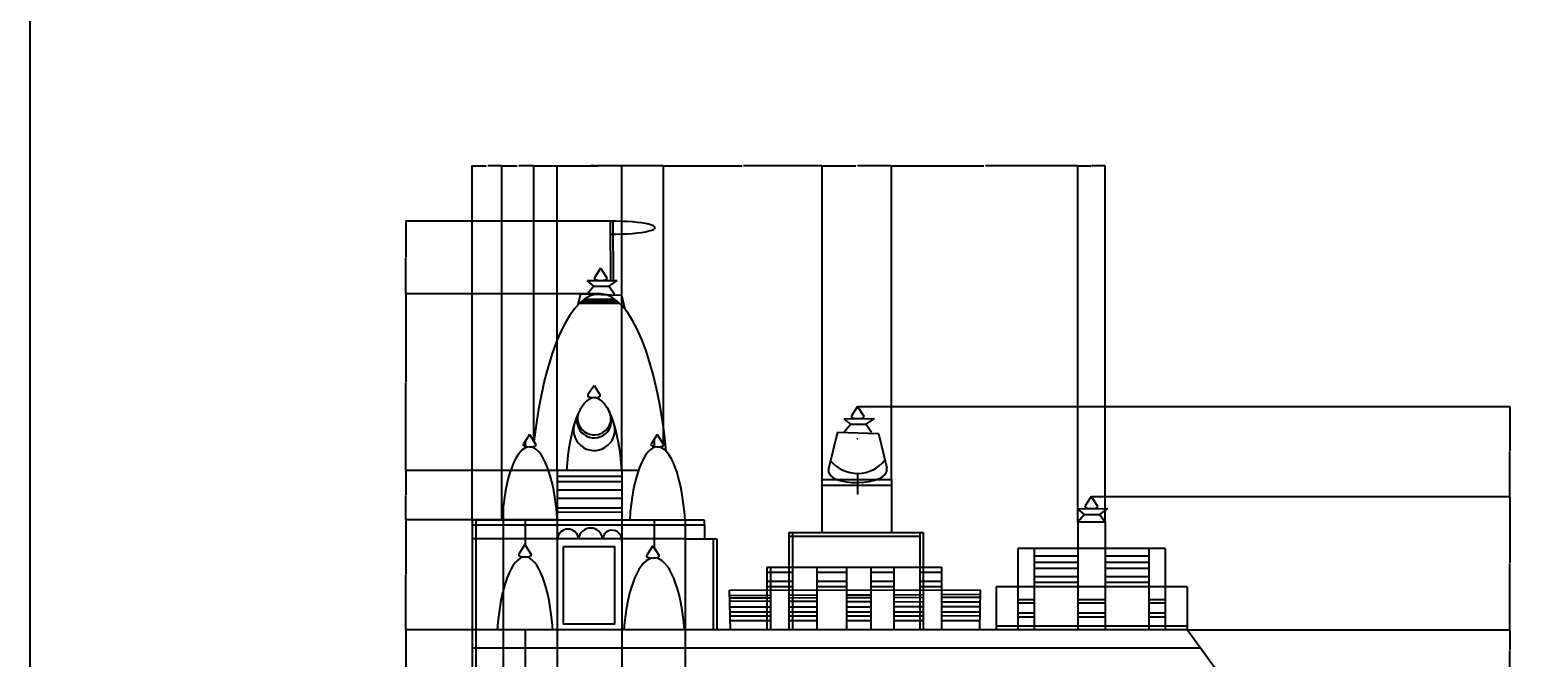
# Model space of a CAD drawing. Units: inches. Extents: x 386 to 107067, y -7 to 96314.
# Tile 2 of 10: x 386 to 1215, y 510 to 855. Entities that reach past the tile are written whole.
import ezdxf

# ---------------------------------------------------------------- set-up
doc = ezdxf.new("R2010")
doc.units = ezdxf.units.IN
doc.layers.add('A-ANNO-DIMS', color=2, linetype='Continuous', lineweight=18)
doc.layers.add('A-ELEV', color=7, linetype='Continuous', lineweight=25)
doc.styles.get("Standard").update_dxf_attribs({"font": 'arial.ttf'})
doc.dimstyles.get("Standard").update_dxf_attribs({"dimtxt": 0.18, "dimasz": 0.18, "dimexe": 0.18, "dimexo": 0.0625, "dimgap": 0.09, "dimtad": 0, "dimtih": 1, "dimtoh": 1, "dimdec": 4, "dimzin": 0, "dimdsep": 46, "dimtxsty": 'Standard', "dimcen": 0.09, "dimadec": 0, "dimazin": 0, "dimtfac": 1, "dimtdec": 4, "dimtofl": 0, "dimtmove": 0, "dimatfit": 3, "dimfxl": 1, "dimtolj": 1, "dimtzin": 0, "dimarcsym": 0})

# ---------------------------------------------------------------- blocks, each defined once
blk = doc.blocks.new('*D56')
at = {"layer": 'A-ANNO-DIMS', "color": 0, "lineweight": -2, "transparency": 16777216}
for p, q in [((628.96, 525.24), (592.35, 525.24)), ((592.53, 525.06), (592.53, 502.06)), ((592.53, 478.69), (592.53, 501.69)), ((728.96, 478.51), (592.35, 478.51))]:
    blk.add_line(p, q, dxfattribs=at)
at = {"layer": 'A-ANNO-DIMS', "color": 0, "transparency": 16777216}
for points in [[(592.5, 525.06), (592.56, 525.06), (592.53, 525.24)], [(592.5, 478.69), (592.56, 478.69), (592.53, 478.51)]]:
    blk.add_solid(points, dxfattribs=at)
at = {"layer": 'Defpoints', "color": 0, "transparency": 16777216}
for p in [(592.53, 525.24), (629.03, 525.24), (729.03, 478.51)]:
    blk.add_point(p, dxfattribs=at)
at = {"layer": 'A-ANNO-DIMS', "color": 0, "transparency": 16777216, "insert": (592.53, 501.88), "char_height": 0.18, "attachment_point": 5}
blk.add_mtext('\\A1;46.73', dxfattribs=at)
blk = doc.blocks.new('*D57')
at = {"layer": 'A-ANNO-DIMS', "color": 0, "lineweight": -2, "transparency": 16777216}
for p, q in [((628.96, 585.71), (592.35, 585.71)), ((592.53, 585.53), (592.53, 555.66)), ((592.53, 525.42), (592.53, 555.3)), ((628.96, 525.24), (592.35, 525.24))]:
    blk.add_line(p, q, dxfattribs=at)
at = {"layer": 'A-ANNO-DIMS', "color": 0, "transparency": 16777216}
for points in [[(592.5, 585.53), (592.56, 585.53), (592.53, 585.71)], [(592.5, 525.42), (592.56, 525.42), (592.53, 525.24)]]:
    blk.add_solid(points, dxfattribs=at)
at = {"layer": 'Defpoints', "color": 0, "transparency": 16777216}
for p in [(592.53, 585.71), (629.03, 585.71), (629.03, 525.24)]:
    blk.add_point(p, dxfattribs=at)
at = {"layer": 'A-ANNO-DIMS', "color": 0, "transparency": 16777216, "insert": (592.53, 555.48), "char_height": 0.18, "attachment_point": 5}
blk.add_mtext('\\A1;60.47', dxfattribs=at)
blk = doc.blocks.new('*D58')
at = {"layer": 'A-ANNO-DIMS', "color": 0, "lineweight": -2, "transparency": 16777216}
for p, q in [((675.71, 612.76), (592.35, 612.76)), ((592.53, 612.58), (592.53, 599.42)), ((592.53, 585.89), (592.53, 599.05)), ((675.71, 585.71), (592.35, 585.71))]:
    blk.add_line(p, q, dxfattribs=at)
at = {"layer": 'A-ANNO-DIMS', "color": 0, "transparency": 16777216}
for points in [[(592.5, 612.58), (592.56, 612.58), (592.53, 612.76)], [(592.5, 585.89), (592.56, 585.89), (592.53, 585.71)]]:
    blk.add_solid(points, dxfattribs=at)
at = {"layer": 'Defpoints', "color": 0, "transparency": 16777216}
for p in [(592.53, 612.76), (675.77, 612.76), (675.77, 585.71)]:
    blk.add_point(p, dxfattribs=at)
at = {"layer": 'A-ANNO-DIMS', "color": 0, "transparency": 16777216, "insert": (592.53, 599.24), "char_height": 0.18, "attachment_point": 5}
blk.add_mtext('\\A1;27.04', dxfattribs=at)
blk = doc.blocks.new('*D59')
at = {"layer": 'A-ANNO-DIMS', "color": 0, "lineweight": -2, "transparency": 16777216}
for p, q in [((699.85, 709.88), (592.35, 709.88)), ((592.53, 709.7), (592.53, 661.5)), ((592.53, 612.94), (592.53, 661.14)), ((675.71, 612.76), (592.35, 612.76))]:
    blk.add_line(p, q, dxfattribs=at)
at = {"layer": 'A-ANNO-DIMS', "color": 0, "transparency": 16777216}
for points in [[(592.5, 709.7), (592.56, 709.7), (592.53, 709.88)], [(592.5, 612.94), (592.56, 612.94), (592.53, 612.76)]]:
    blk.add_solid(points, dxfattribs=at)
at = {"layer": 'Defpoints', "color": 0, "transparency": 16777216}
for p in [(592.53, 709.88), (699.91, 709.88), (675.77, 612.76)]:
    blk.add_point(p, dxfattribs=at)
at = {"layer": 'A-ANNO-DIMS', "color": 0, "transparency": 16777216, "insert": (592.53, 661.32), "char_height": 0.18, "attachment_point": 5}
blk.add_mtext('\\A1;97.12', dxfattribs=at)
blk = doc.blocks.new('*D60')
at = {"layer": 'A-ANNO-DIMS', "color": 0, "lineweight": -2, "transparency": 16777216}
for p, q in [((704.79, 749.79), (592.35, 749.79)), ((592.53, 749.61), (592.53, 730.02)), ((592.53, 710.06), (592.53, 729.65)), ((699.85, 709.88), (592.35, 709.88))]:
    blk.add_line(p, q, dxfattribs=at)
at = {"layer": 'A-ANNO-DIMS', "color": 0, "transparency": 16777216}
for points in [[(592.5, 749.61), (592.56, 749.61), (592.53, 749.79)], [(592.5, 710.06), (592.56, 710.06), (592.53, 709.88)]]:
    blk.add_solid(points, dxfattribs=at)
at = {"layer": 'Defpoints', "color": 0, "transparency": 16777216}
for p in [(592.53, 749.79), (704.85, 749.79), (699.91, 709.88)]:
    blk.add_point(p, dxfattribs=at)
at = {"layer": 'A-ANNO-DIMS', "color": 0, "transparency": 16777216, "insert": (592.53, 729.84), "char_height": 0.18, "attachment_point": 5}
blk.add_mtext('\\A1;39.91', dxfattribs=at)
blk = doc.blocks.new('*D65')
at = {"layer": 'A-ANNO-DIMS', "color": 0, "lineweight": -2, "transparency": 16777216}
for p, q in [((1022.09, 525.24), (1199.71, 525.24)), ((1199.53, 525.06), (1199.53, 514.06)), ((1199.53, 502.69), (1199.53, 513.69)), ((1037.1, 502.51), (1199.71, 502.51))]:
    blk.add_line(p, q, dxfattribs=at)
at = {"layer": 'A-ANNO-DIMS', "color": 0, "transparency": 16777216}
for points in [[(1199.5, 525.06), (1199.56, 525.06), (1199.53, 525.24)], [(1199.5, 502.69), (1199.56, 502.69), (1199.53, 502.51)]]:
    blk.add_solid(points, dxfattribs=at)
at = {"layer": 'Defpoints', "color": 0, "transparency": 16777216}
for p in [(1022.03, 525.24), (1199.53, 525.24), (1037.04, 502.51)]:
    blk.add_point(p, dxfattribs=at)
at = {"layer": 'A-ANNO-DIMS', "color": 0, "transparency": 16777216, "insert": (1199.53, 513.88), "char_height": 0.18, "attachment_point": 5}
blk.add_mtext('\\A1;22.735', dxfattribs=at)
blk = doc.blocks.new('*D66')
at = {"layer": 'A-ANNO-DIMS', "color": 0, "lineweight": -2, "transparency": 16777216}
for p, q in [((969.43, 598.58), (1199.71, 598.58)), ((1199.53, 598.4), (1199.53, 562.09)), ((1199.53, 525.42), (1199.53, 561.73)), ((1022.09, 525.24), (1199.71, 525.24))]:
    blk.add_line(p, q, dxfattribs=at)
at = {"layer": 'A-ANNO-DIMS', "color": 0, "transparency": 16777216}
for points in [[(1199.5, 598.4), (1199.56, 598.4), (1199.53, 598.58)], [(1199.5, 525.42), (1199.56, 525.42), (1199.53, 525.24)]]:
    blk.add_solid(points, dxfattribs=at)
at = {"layer": 'Defpoints', "color": 0, "transparency": 16777216}
for p in [(969.37, 598.58), (1199.53, 598.58), (1022.03, 525.24)]:
    blk.add_point(p, dxfattribs=at)
at = {"layer": 'A-ANNO-DIMS', "color": 0, "transparency": 16777216, "insert": (1199.53, 561.91), "char_height": 0.18, "attachment_point": 5}
blk.add_mtext('\\A1;73.33', dxfattribs=at)
blk = doc.blocks.new('*D67')
at = {"layer": 'A-ANNO-DIMS', "color": 0, "lineweight": -2, "transparency": 16777216}
for p, q in [((840.97, 648.04), (1199.71, 648.04)), ((1199.53, 647.86), (1199.53, 623.49)), ((1199.53, 598.76), (1199.53, 623.13)), ((969.43, 598.58), (1199.71, 598.58))]:
    blk.add_line(p, q, dxfattribs=at)
at = {"layer": 'A-ANNO-DIMS', "color": 0, "transparency": 16777216}
for points in [[(1199.5, 647.86), (1199.56, 647.86), (1199.53, 648.04)], [(1199.5, 598.76), (1199.56, 598.76), (1199.53, 598.58)]]:
    blk.add_solid(points, dxfattribs=at)
at = {"layer": 'Defpoints', "color": 0, "transparency": 16777216}
for p in [(840.91, 648.04), (1199.53, 648.04), (969.37, 598.58)]:
    blk.add_point(p, dxfattribs=at)
at = {"layer": 'A-ANNO-DIMS', "color": 0, "transparency": 16777216, "insert": (1199.53, 623.31), "char_height": 0.18, "attachment_point": 5}
blk.add_mtext('\\A1;49.46', dxfattribs=at)
blk = doc.blocks.new('*D77')
at = {"layer": 'A-ANNO-DIMS', "color": 0, "lineweight": -2, "transparency": 16777216}
for p, q in [((629.03, 585.78), (629.03, 780.47)), ((629.21, 780.29), (636.73, 780.29)), ((645.16, 780.29), (637.64, 780.29)), ((645.34, 585.78), (645.34, 780.47))]:
    blk.add_line(p, q, dxfattribs=at)
at = {"layer": 'A-ANNO-DIMS', "color": 0, "transparency": 16777216}
for points in [[(629.21, 780.32), (629.21, 780.26), (629.03, 780.29)], [(645.16, 780.32), (645.16, 780.26), (645.34, 780.29)]]:
    blk.add_solid(points, dxfattribs=at)
at = {"layer": 'Defpoints', "color": 0, "transparency": 16777216}
for p in [(645.34, 780.29), (629.03, 585.71), (645.34, 585.71)]:
    blk.add_point(p, dxfattribs=at)
at = {"layer": 'A-ANNO-DIMS', "color": 0, "transparency": 16777216, "insert": (637.18, 780.29), "char_height": 0.18, "attachment_point": 5}
blk.add_mtext('\\A1;16.315', dxfattribs=at)
blk = doc.blocks.new('*D78')
at = {"layer": 'A-ANNO-DIMS', "color": 0, "lineweight": -2, "transparency": 16777216}
for p, q in [((645.34, 585.78), (645.34, 780.47)), ((645.52, 780.29), (653.68, 780.29)), ((662.74, 780.29), (654.59, 780.29)), ((662.92, 628.76), (662.92, 780.47))]:
    blk.add_line(p, q, dxfattribs=at)
at = {"layer": 'A-ANNO-DIMS', "color": 0, "transparency": 16777216}
for points in [[(645.52, 780.32), (645.52, 780.26), (645.34, 780.29)], [(662.74, 780.32), (662.74, 780.26), (662.92, 780.29)]]:
    blk.add_solid(points, dxfattribs=at)
at = {"layer": 'Defpoints', "color": 0, "transparency": 16777216}
for p in [(662.92, 780.29), (662.92, 628.7), (645.34, 585.71)]:
    blk.add_point(p, dxfattribs=at)
at = {"layer": 'A-ANNO-DIMS', "color": 0, "transparency": 16777216, "insert": (654.13, 780.29), "char_height": 0.18, "attachment_point": 5}
blk.add_mtext('\\A1;17.582', dxfattribs=at)
blk = doc.blocks.new('*D79')
at = {"layer": 'A-ANNO-DIMS', "color": 0, "lineweight": -2, "transparency": 16777216}
for p, q in [((662.92, 628.76), (662.92, 780.47)), ((663.1, 780.29), (698.14, 780.29)), ((733.96, 780.29), (698.93, 780.29)), ((734.14, 627.23), (734.14, 780.47))]:
    blk.add_line(p, q, dxfattribs=at)
at = {"layer": 'A-ANNO-DIMS', "color": 0, "transparency": 16777216}
for points in [[(663.1, 780.32), (663.1, 780.26), (662.92, 780.29)], [(733.96, 780.32), (733.96, 780.26), (734.14, 780.29)]]:
    blk.add_solid(points, dxfattribs=at)
at = {"layer": 'Defpoints', "color": 0, "transparency": 16777216}
for p in [(734.14, 780.29), (662.92, 628.7), (734.14, 627.16)]:
    blk.add_point(p, dxfattribs=at)
at = {"layer": 'A-ANNO-DIMS', "color": 0, "transparency": 16777216, "insert": (698.53, 780.29), "char_height": 0.18, "attachment_point": 5}
blk.add_mtext('\\A1;71.22', dxfattribs=at)
blk = doc.blocks.new('*D80')
at = {"layer": 'A-ANNO-DIMS', "color": 0, "lineweight": -2, "transparency": 16777216}
for p, q in [((734.14, 627.23), (734.14, 780.47)), ((734.32, 780.29), (777.34, 780.29)), ((821.15, 780.29), (778.13, 780.29)), ((821.33, 607.9), (821.33, 780.47))]:
    blk.add_line(p, q, dxfattribs=at)
at = {"layer": 'A-ANNO-DIMS', "color": 0, "transparency": 16777216}
for points in [[(734.32, 780.32), (734.32, 780.26), (734.14, 780.29)], [(821.15, 780.32), (821.15, 780.26), (821.33, 780.29)]]:
    blk.add_solid(points, dxfattribs=at)
at = {"layer": 'Defpoints', "color": 0, "transparency": 16777216}
for p in [(821.33, 780.29), (734.14, 627.16), (821.33, 607.84)]:
    blk.add_point(p, dxfattribs=at)
at = {"layer": 'A-ANNO-DIMS', "color": 0, "transparency": 16777216, "insert": (777.74, 780.29), "char_height": 0.18, "attachment_point": 5}
blk.add_mtext('\\A1;87.19', dxfattribs=at)
blk = doc.blocks.new('*D81')
at = {"layer": 'A-ANNO-DIMS', "color": 0, "lineweight": -2, "transparency": 16777216}
for p, q in [((821.33, 607.9), (821.33, 780.47)), ((821.51, 780.29), (839.95, 780.29)), ((859.32, 780.29), (840.88, 780.29)), ((859.5, 607.9), (859.5, 780.47))]:
    blk.add_line(p, q, dxfattribs=at)
at = {"layer": 'A-ANNO-DIMS', "color": 0, "transparency": 16777216}
for points in [[(821.51, 780.32), (821.51, 780.26), (821.33, 780.29)], [(859.32, 780.32), (859.32, 780.26), (859.5, 780.29)]]:
    blk.add_solid(points, dxfattribs=at)
at = {"layer": 'Defpoints', "color": 0, "transparency": 16777216}
for p in [(859.5, 780.29), (821.33, 607.84), (859.5, 607.84)]:
    blk.add_point(p, dxfattribs=at)
at = {"layer": 'A-ANNO-DIMS', "color": 0, "transparency": 16777216, "insert": (840.42, 780.29), "char_height": 0.18, "attachment_point": 5}
blk.add_mtext('\\A1;38.165', dxfattribs=at)
blk = doc.blocks.new('*D82')
at = {"layer": 'A-ANNO-DIMS', "color": 0, "lineweight": -2, "transparency": 16777216}
for p, q in [((859.5, 607.9), (859.5, 780.47)), ((859.68, 780.29), (910.31, 780.29)), ((961.85, 780.29), (911.22, 780.29)), ((962.03, 584.41), (962.03, 780.47))]:
    blk.add_line(p, q, dxfattribs=at)
at = {"layer": 'A-ANNO-DIMS', "color": 0, "transparency": 16777216}
for points in [[(859.68, 780.32), (859.68, 780.26), (859.5, 780.29)], [(961.85, 780.32), (961.85, 780.26), (962.03, 780.29)]]:
    blk.add_solid(points, dxfattribs=at)
at = {"layer": 'Defpoints', "color": 0, "transparency": 16777216}
for p in [(962.03, 780.29), (859.5, 607.84), (962.03, 584.35)]:
    blk.add_point(p, dxfattribs=at)
at = {"layer": 'A-ANNO-DIMS', "color": 0, "transparency": 16777216, "insert": (910.76, 780.29), "char_height": 0.18, "attachment_point": 5}
blk.add_mtext('\\A1;102.53', dxfattribs=at)
blk = doc.blocks.new('*D83')
at = {"layer": 'A-ANNO-DIMS', "color": 0, "lineweight": -2, "transparency": 16777216}
for p, q in [((962.03, 584.41), (962.03, 780.47)), ((962.21, 780.29), (969.31, 780.29)), ((976.85, 780.29), (969.74, 780.29)), ((977.03, 584.41), (977.03, 780.47))]:
    blk.add_line(p, q, dxfattribs=at)
at = {"layer": 'A-ANNO-DIMS', "color": 0, "transparency": 16777216}
for points in [[(962.21, 780.32), (962.21, 780.26), (962.03, 780.29)], [(976.85, 780.32), (976.85, 780.26), (977.03, 780.29)]]:
    blk.add_solid(points, dxfattribs=at)
at = {"layer": 'Defpoints', "color": 0, "transparency": 16777216}
for p in [(977.03, 780.29), (962.03, 584.35), (977.03, 584.35)]:
    blk.add_point(p, dxfattribs=at)
at = {"layer": 'A-ANNO-DIMS', "color": 0, "transparency": 16777216, "insert": (969.53, 780.29), "char_height": 0.18, "attachment_point": 5}
blk.add_mtext('\\A1;15', dxfattribs=at)
blk = doc.blocks.new('*D84')
at = {"layer": 'A-ANNO-DIMS', "color": 0, "lineweight": -2, "transparency": 16777216}
for p, q in [((675.77, 612.82), (675.77, 780.47)), ((675.95, 780.29), (693.06, 780.29)), ((711.09, 780.29), (693.98, 780.29)), ((711.27, 612.82), (711.27, 780.47))]:
    blk.add_line(p, q, dxfattribs=at)
at = {"layer": 'A-ANNO-DIMS', "color": 0, "transparency": 16777216}
for points in [[(675.95, 780.32), (675.95, 780.26), (675.77, 780.29)], [(711.09, 780.32), (711.09, 780.26), (711.27, 780.29)]]:
    blk.add_solid(points, dxfattribs=at)
at = {"layer": 'Defpoints', "color": 0, "transparency": 16777216}
for p in [(711.27, 780.29), (675.77, 612.76), (711.27, 612.76)]:
    blk.add_point(p, dxfattribs=at)
at = {"layer": 'A-ANNO-DIMS', "color": 0, "transparency": 16777216, "insert": (693.52, 780.29), "char_height": 0.18, "attachment_point": 5}
blk.add_mtext('\\A1;35.496', dxfattribs=at)
blk = doc.blocks.new('*D92')
at = {"layer": 'A-ANNO-DIMS', "color": 0, "lineweight": -2, "transparency": 16777216}
for p, q in [((840.73, 630.26), (840.91, 630.26)), ((840.82, 630.17), (840.82, 630.35)), ((841.11, 599.8), (841, 611.04)), ((841.29, 599.8), (841.11, 599.8))]:
    blk.add_line(p, q, dxfattribs=at)
at = {"layer": 'A-ANNO-DIMS', "color": 0, "transparency": 16777216}
blk.add_solid([(841.03, 611.04), (840.97, 611.04), (841, 611.22)], dxfattribs=at)
at = {"layer": 'Defpoints', "color": 0, "transparency": 16777216}
for p in [(840.82, 630.26), (841, 611.22)]:
    blk.add_point(p, dxfattribs=at)
at = {"layer": 'A-ANNO-DIMS', "color": 0, "transparency": 16777216, "insert": (841.76, 599.8), "char_height": 0.18, "attachment_point": 5}
blk.add_mtext('\\A1;R19.04', dxfattribs=at)

msp = doc.modelspace()

# ---------------------------------------------------------------- linework, layer by layer
at = {"layer": 'A-ELEV'}
for p, q in [((704.8536, 749.7917), (704.9724, 717.2635)), ((704.8536, 749.7917), (706.394, 749.7917)), ((706.394, 749.7917), (706.5128, 717.2692)), ((699.5858, 723.9778), (696.1948, 718.7355)), ((699.5858, 723.9778), (702.9769, 718.6076)), ((692.2048, 717.2169), (708.7758, 717.2774)), ((695.8991, 714.1217), (692.2048, 717.2169)), ((695.8991, 714.1217), (692.2387, 709.7528)), ((695.8991, 714.1217), (704.2155, 714.1217)), ((704.2155, 714.1217), (708.7758, 717.2774)), ((704.2155, 714.1217), (707.2387, 709.7528)), ((688.5858, 709.8864), (687.1082, 703.8169)), ((688.1023, 704.8132), (710.0986, 704.656)), ((688.5858, 709.8864), (711.0341, 709.0657)), ((689.0115, 705.6421), (709.2459, 705.4488)), ((689.9002, 706.3779), (708.1231, 706.3891)), ((690.6702, 706.957), (707.4109, 706.9256)), ((711.0341, 709.0657), (712.8802, 701.5787)), ((695.9971, 659.5746), (692.6061, 654.3323)), ((695.9971, 659.5746), (699.3882, 654.2045)), ((840.906, 648.0385), (837.515, 642.7962)), ((840.906, 648.0385), (844.2971, 642.6683)), ((833.5251, 641.2776), (850.096, 641.3382)), ((837.2193, 638.1824), (833.5251, 641.2776)), ((845.5357, 638.1824), (850.096, 641.3382)), ((660.5011, 632.5327), (657.1101, 627.2904)), ((660.5011, 632.5327), (663.8922, 627.1625)), ((730.7531, 632.5327), (727.3621, 627.2904)), ((730.7531, 632.5327), (734.1442, 627.1625)), ((829.906, 633.9471), (824.9784, 613.7052)), ((829.906, 633.9471), (852.3543, 633.1264)), ((837.2193, 638.1824), (833.5589, 633.8135)), ((837.2193, 638.1824), (845.5357, 638.1824)), ((845.5357, 638.1824), (848.5589, 633.8135)), ((852.3543, 633.1264), (857.0082, 614.2523)), ((658.0252, 628.7051), (658.0252, 625.1267)), ((729.0252, 629.8614), (729.0252, 625.4652)), ((720.3574, 612.7565), (671.0082, 612.7565)), ((675.7732, 612.7565), (675.7732, 451.5096)), ((675.7732, 609.7656), (711.2692, 609.7656)), ((711.2692, 606.5849), (675.7732, 606.5849)), ((711.2692, 612.7565), (711.2692, 322.5096)), ((821.3331, 578.7205), (821.3331, 607.8412)), ((821.3331, 607.8412), (859.4982, 607.8412)), ((859.4982, 607.8412), (859.4982, 578.7205)), ((675.7732, 602.1925), (711.2692, 602.1925)), ((711.2692, 597.4972), (675.7732, 597.4972)), ((821.3331, 604.8412), (859.4982, 604.8412)), ((969.3723, 598.5774), (965.9813, 593.3351)), ((969.3723, 598.5774), (972.7634, 593.2072)), ((646.0252, 593.3749), (646.0252, 274.5096)), ((675.7732, 592.3476), (711.2692, 592.3476)), ((711.2692, 589.9241), (675.7732, 589.7442)), ((961.9913, 591.8165), (978.5623, 591.877)), ((965.6856, 588.7213), (961.9913, 591.8165)), ((965.6856, 588.7213), (962.0252, 584.3524)), ((965.6856, 588.7213), (974.002, 588.7213)), ((974.002, 588.7213), (978.5623, 591.877)), ((974.002, 588.7213), (977.0252, 584.3524)), ((629.0252, 585.7146), (629.0252, 502.5096)), ((629.0252, 585.7146), (629.0252, 502.5096)), ((629.0252, 585.7146), (746.0252, 585.7146)), ((629.0252, 583.0118), (746.0252, 583.0118)), ((631.0252, 585.7146), (631.0252, 502.5096)), ((658.0252, 585.7146), (658.0252, 571.9741)), ((675.7732, 585.7146), (711.2692, 585.7146)), ((729.0252, 585.7146), (729.0252, 570.3474)), ((746.0252, 585.7146), (746.0252, 525.2442)), ((746.0252, 585.7146), (756.4861, 585.7146)), ((746.0252, 583.0118), (756.6362, 583.0118)), ((756.4861, 585.7146), (756.4861, 583.0118)), ((756.6362, 583.0118), (756.6362, 575.3263)), ((962.0252, 584.3524), (962.0252, 525.2442)), ((977.0252, 584.3524), (962.0252, 584.3524)), ((977.0252, 584.3524), (977.0252, 525.2442)), ((746.0252, 575.3263), (629.0252, 575.3263)), ((657.9695, 572.0623), (654.5785, 566.82)), ((657.9695, 572.0623), (661.3606, 566.6921)), ((746.0252, 575.3263), (763.5261, 575.3263)), ((761.3925, 575.3263), (761.3925, 525.2442)), ((763.5261, 575.3263), (763.5261, 525.2442)), ((803.0252, 578.7205), (803.0252, 525.2442)), ((803.0252, 578.7205), (875.0252, 578.7205)), ((803.0252, 576.7205), (875.0252, 576.7205)), ((805.0252, 578.7205), (805.0252, 525.2442)), ((875.0252, 578.7205), (875.0252, 525.2442)), ((875.0252, 578.7205), (877.0252, 578.7205)), ((877.0252, 578.7205), (877.0252, 525.2442)), ((728.3139, 571.4737), (724.923, 566.2314)), ((728.3139, 571.4737), (731.7051, 566.1036)), ((729.0252, 564.7745), (729.0252, 564.7473)), ((929.0252, 569.9003), (929.0252, 525.2442)), ((1010.0252, 569.9003), (929.0252, 569.9003)), ((938.0252, 569.9003), (938.0252, 525.2442)), ((938.0252, 565.8324), (962.0252, 565.8324)), ((977.0252, 565.8324), (1001.0252, 565.8324)), ((1001.0252, 569.9003), (1001.0252, 525.2442)), ((1010.0252, 569.9003), (1010.0252, 525.2442)), ((791.0252, 559.7024), (791.0252, 525.2442)), ((791.0252, 559.7024), (887.0252, 559.7024)), ((805.0252, 556.8053), (791.0252, 556.8053)), ((793.0252, 559.7024), (793.0252, 525.2442)), ((818.4886, 559.7024), (818.4886, 525.2442)), ((834.7141, 556.8053), (818.4886, 556.8053)), ((834.7141, 559.7024), (834.7141, 525.2442)), ((848.2048, 559.7024), (848.2048, 525.2442)), ((860.7841, 556.8053), (848.2048, 556.8053)), ((860.7841, 559.7024), (860.7841, 525.2442)), ((887.0252, 556.8053), (875.0252, 556.8053)), ((887.0252, 559.7024), (887.0252, 525.2442)), ((938.0252, 562.515), (962.0252, 562.515)), ((962.0252, 559.0468), (938.0252, 559.0468)), ((977.0252, 562.515), (1001.0252, 562.515)), ((1001.0252, 559.0468), (977.0252, 559.0468)), ((770.3702, 547.0345), (908.4441, 547.185)), ((791.0252, 551.9823), (805.0252, 551.9823)), ((791.0252, 549.1438), (805.0252, 549.1438)), ((818.4886, 551.9823), (834.7141, 551.9823)), ((818.4886, 549.1438), (834.7141, 549.1438)), ((848.2048, 551.9823), (860.7841, 551.9823)), ((848.2048, 549.1438), (860.7841, 549.1438)), ((875.0252, 551.9823), (887.0252, 551.9823)), ((875.0252, 549.1438), (887.0252, 549.1438)), ((908.1409, 525.2442), (908.4441, 547.185)), ((917.0252, 548.8243), (917.0252, 525.2442)), ((1022.0252, 548.8243), (917.0252, 548.8243)), ((938.0252, 554.5231), (962.0252, 554.5231)), ((962.0252, 551.2057), (938.0252, 551.2057)), ((977.0252, 554.5231), (1001.0252, 554.5231)), ((1001.0252, 551.2057), (977.0252, 551.2057)), ((1022.0252, 548.8243), (1022.0252, 525.2442)), ((771.0601, 525.2442), (770.3702, 547.0345)), ((770.4597, 544.2092), (793.0252, 544.3016)), ((793.0252, 542.7173), (770.5092, 542.6456)), ((793.0252, 540.8725), (770.5624, 540.9655)), ((803.0252, 544.3425), (818.4886, 544.4058)), ((818.4886, 542.7984), (803.0252, 542.7492)), ((818.4886, 540.767), (803.0252, 540.8311)), ((834.7141, 544.4723), (848.2048, 544.5275)), ((848.2048, 542.8931), (834.7141, 542.8501)), ((848.2048, 540.644), (834.7141, 540.6998)), ((860.7841, 544.579), (877.0252, 544.6455)), ((877.0252, 542.9849), (860.7841, 542.9332)), ((877.0252, 540.5246), (860.7841, 540.5919)), ((887.0252, 544.6865), (908.4107, 544.774)), ((908.3874, 543.0848), (887.0252, 543.0168)), ((908.3503, 540.3949), (887.0252, 540.4832)), ((929.0252, 541.8566), (938.0252, 541.8566)), ((938.0252, 539.8963), (929.0252, 539.8963)), ((962.0252, 541.8566), (977.0252, 541.8566)), ((977.0252, 539.8963), (962.0252, 539.8963)), ((1001.0252, 541.8566), (1010.0252, 541.8566)), ((1010.0252, 539.8963), (1001.0252, 539.8963)), ((770.6585, 537.9278), (793.0252, 537.9441)), ((770.7442, 535.2221), (793.0252, 535.2208)), ((793.0252, 532.7842), (770.8219, 532.768)), ((803.0252, 537.9514), (818.4886, 537.9627)), ((803.0252, 535.2202), (818.4886, 535.2193)), ((818.4886, 532.8028), (803.0252, 532.7915)), ((834.7141, 537.9745), (848.2048, 537.9843)), ((834.7141, 535.2183), (848.2048, 535.2175)), ((848.2048, 532.8246), (834.7141, 532.8147)), ((860.7841, 537.9935), (877.0252, 538.0053)), ((860.7841, 535.2168), (877.0252, 535.2158)), ((877.0252, 532.8456), (860.7841, 532.8338)), ((887.0252, 538.0126), (908.3176, 538.0281)), ((887.0252, 535.2153), (908.2787, 535.214)), ((908.2463, 532.8685), (887.0252, 532.853)), ((929.0252, 534.6186), (938.0252, 534.6186)), ((938.0252, 532.2059), (929.0252, 532.2059)), ((962.0252, 534.6186), (977.0252, 534.6186)), ((977.0252, 532.2059), (962.0252, 532.2059)), ((1001.0252, 534.6186), (1010.0252, 534.6186)), ((1010.0252, 532.2059), (1001.0252, 532.2059)), ((1022.0252, 525.2442), (629.0252, 525.2442)), ((658.0252, 525.2442), (658.0252, 274.5096)), ((746.0252, 525.2442), (746.0252, 395.5096)), ((770.8992, 530.3255), (793.0252, 530.3398)), ((803.0252, 530.3463), (818.4886, 530.3563)), ((834.7141, 530.3668), (848.2048, 530.3755)), ((860.7841, 530.3837), (877.0252, 530.3942)), ((887.0252, 530.4006), (908.2124, 530.4144)), ((917.0252, 527.5314), (1022.0252, 527.5314)), ((1037.0367, 504.5096), (1022.0252, 525.2442)), ((1029.265, 515.2442), (629.0252, 515.2442))]:
    msp.add_line(p, q, dxfattribs=at)
for points in [[(385.946, 1737.774), (1886.0535, 1737.774), (1886.0535, -7.0679), (385.946, -7.0679)], [(679.2711, 571.129), (707.2736, 571.129), (707.2736, 528.4231), (679.2711, 528.4231)]]:
    msp.add_lwpolyline(points, close=True, dxfattribs=at)
for centre, radius, start, end in [((696.0843, 641.5613), 9.1685, 164.4712011, 41.7119135), ((696.0676, 635.2088), 11.404, 166.6176048, 23.8998163), ((696.0601, 640.2862), 9.5667, 157.0539711, 28.6245156), ((840.8192, 630.262), 19.0416, 219.2592308, 322.4733116), ((681.6492, 574.6836), 5.911, 6.2415855, 173.7584145), ((694.116, 574.5576), 6.6354, 6.6520305, 173.3479695), ((705.988, 574.6416), 5.3254, 352.613369, 172.613369)]:
    msp.add_arc(centre, radius, start, end, dxfattribs=at)
for centre, major_axis, ratio, start_param, end_param in [((706.4069, 746.2524), (23.099, 0), 0.15322324, 4.64621231, 7.92127769), ((699.0188, 585.8762), (0, 124.0382), 0.31007336, 5.01850833, 7.50149618), ((696.0528, 602.7565), (0, 50.0821), 0.31007336, 4.91341231, 7.6529583), ((660.5568, 575.7146), (0, 50.0821), 0.31007336, 4.91341231, 7.6529583), ((699.0188, 585.8762), (0, 124.0382), 0.31007336, 7.52486979, 7.52987155), ((730.8088, 575.7146), (0, 50.0821), 0.31007336, 4.91341231, 7.6529583), ((658.0252, 515.2442), (0, 50.0821), 0.31007336, 4.91341231, 7.6529583), ((729.0252, 515.2442), (0, 49.5304), 0.34322375, 4.91568271, 7.65068791)]:
    msp.add_ellipse(centre, major_axis=major_axis, ratio=ratio, start_param=start_param, end_param=end_param, dxfattribs=at)
for points in [[(696.1948, 718.7355), (694.9668, 716.8369), (704.1842, 716.6958), (702.9769, 718.6076)], [(692.6061, 654.3323), (691.3781, 652.4338), (700.5955, 652.2926), (699.3882, 654.2045)], [(837.515, 642.7962), (836.287, 640.8977), (845.5044, 640.7565), (844.2971, 642.6683)], [(657.1101, 627.2904), (655.8821, 625.3919), (665.0995, 625.2507), (663.8922, 627.1625)], [(727.3621, 627.2904), (726.1341, 625.3919), (735.3515, 625.2507), (734.1442, 627.1625)], [(824.9784, 613.7052), (822.4527, 603.3301), (859.5646, 603.8847), (857.0082, 614.2523)], [(965.9813, 593.3351), (964.7532, 591.4365), (973.9706, 591.2954), (972.7634, 593.2072)], [(654.5785, 566.82), (653.3505, 564.9215), (662.5679, 564.7803), (661.3606, 566.6921)], [(724.923, 566.2314), (723.6949, 564.3329), (732.9123, 564.1917), (731.7051, 566.1036)]]:
    msp.add_open_spline(points, degree=3, dxfattribs=at)

# ---------------------------------------------------------------- dimensions: what is measured, and where the dimension line sits
at = {"layer": 'A-ANNO-DIMS'}
for base, p1, p2, override, picture, middle in [((645.3404, 780.2917), (629.0252, 585.7146), (645.3404, 585.7146), {"dimdec": 3, "dimlfac": 1, "dimrnd": 0, "dimzin": 0, "dimdsep": 46, "dimlunit": 2}, '*D77', (637.1828, 780.2917)), ((662.9225, 780.2917), (645.3404, 585.7146), (662.9225, 628.6981), {"dimdec": 3, "dimlfac": 1, "dimrnd": 0, "dimzin": 0, "dimdsep": 46, "dimlunit": 2}, '*D78', (654.1314, 780.2917)), ((734.1442, 780.2917), (662.9225, 628.6981), (734.1442, 627.1625), {"dimdec": 2, "dimlfac": 1, "dimrnd": 0, "dimzin": 0, "dimdsep": 46, "dimlunit": 2}, '*D79', (698.5334, 780.2917)), ((711.2692, 780.2917), (675.7732, 612.7565), (711.2692, 612.7565), {"dimdec": 3, "dimlfac": 1, "dimrnd": 0, "dimzin": 0, "dimdsep": 46, "dimlunit": 2}, '*D84', (693.5212, 780.2917)), ((821.3331, 780.2917), (734.1442, 627.1625), (821.3331, 607.8412), {"dimdec": 2, "dimlfac": 1, "dimrnd": 0, "dimzin": 0, "dimdsep": 46, "dimlunit": 2}, '*D80', (777.7386, 780.2917)), ((859.4982, 780.2917), (821.3331, 607.8412), (859.4982, 607.8412), {"dimdec": 3, "dimlfac": 1, "dimrnd": 0, "dimzin": 0, "dimdsep": 46, "dimlunit": 2}, '*D81', (840.4156, 780.2917)), ((962.0252, 780.2917), (859.4982, 607.8412), (962.0252, 584.3524), {"dimdec": 2, "dimlfac": 1, "dimrnd": 0, "dimzin": 0, "dimdsep": 46, "dimlunit": 2}, '*D82', (910.7617, 780.2917)), ((977.0252, 780.2917), (962.0252, 584.3524), (977.0252, 584.3524), {"dimdec": 0, "dimlfac": 1, "dimrnd": 0, "dimzin": 0, "dimdsep": 46, "dimlunit": 2}, '*D83', (969.5252, 780.2917))]:
    dim = msp.add_linear_dim(base=base, p1=p1, p2=p2, dimstyle='Standard', override=override, dxfattribs=at)
    dim.commit()
    dim.dimension.update_dxf_attribs({"geometry": picture, "text_midpoint": middle})
for base, p1, p2, override, picture, middle in [((592.5252, 749.7917), (699.9103, 709.8811), (704.8536, 749.7917), {"dimdec": 2, "dimlfac": 1, "dimrnd": 0, "dimzin": 0, "dimdsep": 46, "dimlunit": 2}, '*D60', (592.5252, 729.8364)), ((592.5252, 709.8811), (675.7732, 612.7565), (699.9103, 709.8811), {"dimdec": 2, "dimlfac": 1, "dimrnd": 0, "dimzin": 0, "dimdsep": 46, "dimlunit": 2}, '*D59', (592.5252, 661.3188)), ((1199.5252, 648.0385), (969.3723, 598.5774), (840.906, 648.0385), {"dimdec": 2, "dimlfac": 1, "dimrnd": 0, "dimzin": 0, "dimdsep": 46, "dimlunit": 2}, '*D67', (1199.5252, 623.3079)), ((592.5252, 612.7565), (675.7732, 585.7146), (675.7732, 612.7565), {"dimdec": 2, "dimlfac": 1, "dimrnd": 0, "dimzin": 0, "dimdsep": 46, "dimlunit": 2}, '*D58', (592.5252, 599.2355)), ((1199.5252, 598.5774), (1022.0252, 525.2442), (969.3723, 598.5774), {"dimdec": 2, "dimlfac": 1, "dimrnd": 0, "dimzin": 0, "dimdsep": 46, "dimlunit": 2}, '*D66', (1199.5252, 561.9108)), ((592.5252, 585.7146), (629.0252, 525.2442), (629.0252, 585.7146), {"dimdec": 2, "dimlfac": 1, "dimrnd": 0, "dimzin": 0, "dimdsep": 46, "dimlunit": 2}, '*D57', (592.5252, 555.4794)), ((592.5252, 525.2442), (729.0252, 478.5096), (629.0252, 525.2442), {"dimdec": 2, "dimlfac": 1, "dimrnd": 0, "dimzin": 0, "dimdsep": 46, "dimlunit": 2}, '*D56', (592.5252, 501.8769)), ((1199.5252, 525.2442), (1037.0367, 502.5096), (1022.0252, 525.2442), {"dimdec": 3, "dimlfac": 1, "dimrnd": 0, "dimzin": 0, "dimdsep": 46, "dimlunit": 2}, '*D65', (1199.5252, 513.8769))]:
    dim = msp.add_linear_dim(base=base, p1=p1, p2=p2, angle=90, dimstyle='Standard', override=override, dxfattribs=at)
    dim.commit()
    dim.dimension.update_dxf_attribs({"geometry": picture, "text_midpoint": middle})
dim = msp.add_radius_dim(center=(840.8192, 630.262), mpoint=(840.9979, 611.2212), dimstyle='Standard', override={"dimdec": 2, "dimlfac": 1, "dimrnd": 0, "dimzin": 0, "dimdsep": 46, "dimlunit": 2}, dxfattribs=at)
dim.commit()
dim.dimension.update_dxf_attribs({"geometry": '*D92', "text_midpoint": (841.7646, 599.7967), "dimtype": 164})

doc.saveas('drawing.dxf')
